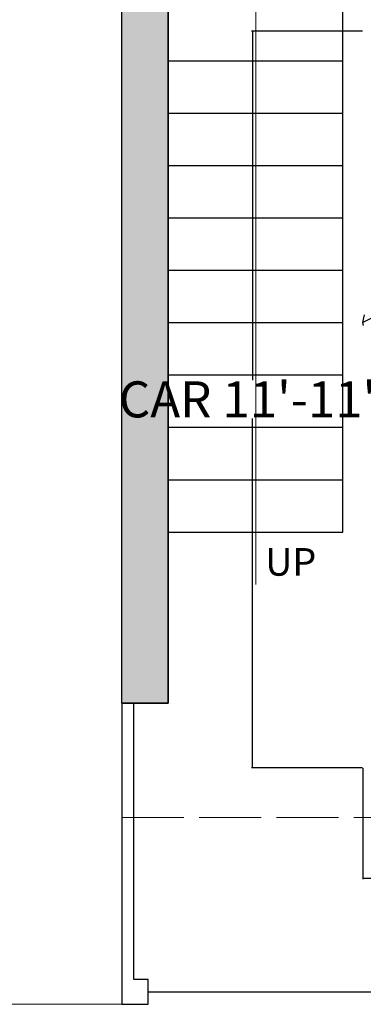
# Model space of a CAD drawing. Units: inches. Extents: x 0 to 4258, y 0 to 3769.
# Tile 3 of 30: x 3659 to 3726, y 2937 to 3128. Entities that reach past the tile are written whole.
import ezdxf

# ---------------------------------------------------------------- set-up
doc = ezdxf.new("R2010")
doc.units = ezdxf.units.IN
doc.header["$MEASUREMENT"] = 0
doc.linetypes.add('ACAD_ISO02W100', pattern=[15, 12, -3])
doc.layers.get('0').update_dxf_attribs({"color": 16})
for name, color, linetype, lineweight in [('A-ANNO-DIMS', 250, 'Continuous', 18), ('A-ANNO-SYMB', 250, 'Continuous', 18), ('A-ANNO-TEXT', 250, 'Continuous', 18), ('A-FLOR-OVHD', 150, 'ACAD_ISO02W100', 13), ('A-FLOR-STRS', 150, 'Continuous', 25), ('A-WALL-PATT', 16, 'Continuous', 13), ('C-PKNG-VEHI', 8, 'Continuous', 18), ('C-PROP', 150, 'Continuous', 25), ('C-ROAD', 250, 'Continuous', 18), ('walls', 251, 'Continuous', 35)]:
    doc.layers.add(name, color=color, linetype=linetype, lineweight=lineweight)
doc.layers.add('Edges', color=250, linetype='Continuous')
doc.styles.get("Standard").update_dxf_attribs({"font": 'arial.ttf'})
doc.dimstyles.get("Standard").update_dxf_attribs({"dimtxt": 7, "dimasz": 0.18, "dimexe": 0.18, "dimexo": 0.0625, "dimgap": 0.09, "dimtad": 0, "dimtih": 1, "dimtoh": 1, "dimzin": 0, "dimdsep": 46, "dimlunit": 3, "dimtxsty": 'Standard', "dimcen": 0.09, "dimadec": 0, "dimazin": 0, "dimtfac": 1, "dimtofl": 0, "dimtmove": 0, "dimatfit": 3, "dimfxl": 1, "dimtolj": 1, "dimtzin": 0, "dimarcsym": 0})

# ---------------------------------------------------------------- blocks, each defined once
blk = doc.blocks.new('Nissan Qashqai pl')
at = {"layer": 'Edges'}
for p, q in [((8.8918, 11.0997), (9.0186, 10.8486)), ((9.0186, 10.8486), (8.9731, 10.8577)), ((9.0374, 10.8517), (9.0186, 10.8486))]:
    blk.add_line(p, q, dxfattribs=at)
blk = doc.blocks.new('car')
blk.add_blockref('Nissan Qashqai pl', (-9.7433, -11.9151))
blk = doc.blocks.new('*D66')
at = {"layer": 'A-ANNO-DIMS', "color": 0, "lineweight": -2, "transparency": 16777216}
for p, q in [((3725.52, 3125.85), (3703.94, 3125.85)), ((3704.12, 3125.67), (3704.12, 3058.01)), ((3704.12, 2982.94), (3704.12, 3050.59)), ((3725.52, 2982.76), (3703.94, 2982.76))]:
    blk.add_line(p, q, dxfattribs=at)
at = {"layer": 'A-ANNO-DIMS', "color": 0, "transparency": 16777216}
for points in [[(3704.09, 3125.67), (3704.15, 3125.67), (3704.12, 3125.85)], [(3704.09, 2982.94), (3704.15, 2982.94), (3704.12, 2982.76)]]:
    blk.add_solid(points, dxfattribs=at)
at = {"layer": 'Defpoints', "color": 0, "transparency": 16777216}
for p in [(3725.58, 3125.85), (3704.12, 2982.76), (3725.58, 2982.76)]:
    blk.add_point(p, dxfattribs=at)
at = {"layer": 'A-ANNO-DIMS', "color": 0, "transparency": 16777216, "insert": (3704.12, 3054.3), "char_height": 7, "attachment_point": 5}
blk.add_mtext('\\A1;CAR 11\'-11"', dxfattribs=at)
blk = doc.blocks.new('*D67')
at = {"layer": 'A-ANNO-DIMS', "color": 0, "lineweight": -2, "transparency": 16777216}
for p, q in [((3725.58, 2982.69), (3725.58, 2961.11)), ((3795.71, 2982.69), (3795.71, 2961.11)), ((3725.76, 2961.29), (3748.53, 2961.29)), ((3795.53, 2961.29), (3772.76, 2961.29))]:
    blk.add_line(p, q, dxfattribs=at)
at = {"layer": 'A-ANNO-DIMS', "color": 0, "transparency": 16777216}
for points in [[(3725.76, 2961.32), (3725.76, 2961.26), (3725.58, 2961.29)], [(3795.53, 2961.32), (3795.53, 2961.26), (3795.71, 2961.29)]]:
    blk.add_solid(points, dxfattribs=at)
at = {"layer": 'Defpoints', "color": 0, "transparency": 16777216}
for p in [(3725.58, 2982.76), (3795.71, 2982.76), (3795.71, 2961.29)]:
    blk.add_point(p, dxfattribs=at)
at = {"layer": 'A-ANNO-DIMS', "color": 0, "transparency": 16777216, "insert": (3760.65, 2961.29), "char_height": 7, "attachment_point": 5}
blk.add_mtext('\\A1;5\'-10"', dxfattribs=at)

msp = doc.modelspace()

# ---------------------------------------------------------------- hatches: boundary and pattern name
at = {"layer": 'A-WALL-PATT'}
h = msp.add_hatch(color=256, dxfattribs=at)
h.dxf.hatch_style = 1
h.paths.add_polyline_path([(3687.804, 3163.293), (3678.804, 3163.293), (3678.804, 2995.293), (3687.804, 2995.293)])
h.paths.add_polyline_path([(3973.039, 3461.793), (3866.304, 3461.793), (3866.304, 3457.293), (3973.039, 3457.293)])
h.paths.add_polyline_path([(4034.304, 3461.793), (4016.474, 3461.793), (4016.474, 3457.293), (4034.304, 3457.293)])

# ---------------------------------------------------------------- linework, layer by layer
at = {"layer": 'A-ANNO-SYMB'}
msp.add_line((3704.8, 3146.777), (3704.8, 3018.327), dxfattribs=at)
at = {"layer": 'A-FLOR-OVHD'}
msp.add_line((3678.804, 2973.052), (3832.744, 2973.052), dxfattribs=at)
at = {"layer": 'A-FLOR-STRS'}
for p, q in [((3721.668, 3028.53), (3721.668, 3163.293)), ((3687.804, 3120.088), (3721.668, 3120.088)), ((3687.804, 3109.915), (3721.668, 3109.915)), ((3687.804, 3099.742), (3721.668, 3099.742)), ((3687.804, 3089.569), (3721.668, 3089.569)), ((3687.804, 3079.396), (3721.668, 3079.396)), ((3687.804, 3069.223), (3721.668, 3069.223)), ((3687.804, 3059.049), (3721.668, 3059.049)), ((3687.804, 3048.876), (3721.668, 3048.876)), ((3687.804, 3038.703), (3721.668, 3038.703)), ((3687.804, 3028.53), (3721.668, 3028.53))]:
    msp.add_line(p, q, dxfattribs=at)
at = {"layer": 'C-PROP'}
for p, q in [((3678.804, 2995.293), (3678.804, 3656.793)), ((3678.804, 2995.293), (3678.804, 2936.793)), ((3681.095, 2941.629), (3681.095, 2995.293)), ((3683.892, 2941.629), (3681.095, 2941.629)), ((3683.892, 2936.793), (3683.892, 2941.629)), ((3683.892, 2939.211), (3766.077, 2939.211)), ((3678.804, 2936.793), (3683.892, 2936.793))]:
    msp.add_line(p, q, dxfattribs=at)
at = {"layer": 'C-ROAD'}
msp.add_line((3678.804, 2936.793), (3596.728, 2936.793), dxfattribs=at)
at = {"layer": 'walls'}
for p, q in [((3687.804, 2995.293), (3687.804, 3163.293)), ((3678.804, 2995.293), (3687.804, 2995.293))]:
    msp.add_line(p, q, dxfattribs=at)

# ---------------------------------------------------------------- block references
at = {"layer": 'C-PKNG-VEHI', "xscale": 32.66500240257601, "yscale": 32.66500240257601, "zscale": 32.66500240257601, "rotation": 270}
msp.add_blockref('car', (3760.419, 3045.57), dxfattribs=at)

# ---------------------------------------------------------------- texts
at = {"layer": 'A-ANNO-TEXT'}
msp.add_text('UP', height=5.3626, dxfattribs=at).set_placement((3706.607, 3020.049))

# ---------------------------------------------------------------- dimensions: what is measured, and where the dimension line sits
at = {"layer": 'A-ANNO-DIMS'}
dim = msp.add_linear_dim(base=(3704.116, 2982.755), p1=(3725.58, 3125.846), p2=(3725.58, 2982.755), angle=270, text='CAR <>', dimstyle='Standard', override={"dimdec": 1, "dimlfac": 1, "dimrnd": 0, "dimzin": 1, "dimdsep": 46, "dimlunit": 4, "dimfrac": 2}, dxfattribs=at)
dim.commit()
dim.dimension.update_dxf_attribs({"geometry": '*D66', "text_midpoint": (3704.116, 3054.301)})
dim = msp.add_linear_dim(base=(3795.713, 2961.292), p1=(3725.58, 2982.755), p2=(3795.713, 2982.755), dimstyle='Standard', override={"dimdec": 1, "dimlfac": 1, "dimrnd": 0, "dimzin": 1, "dimdsep": 46, "dimlunit": 4, "dimfrac": 2}, dxfattribs=at)
dim.commit()
dim.dimension.update_dxf_attribs({"geometry": '*D67', "text_midpoint": (3760.646, 2961.292)})

doc.saveas('drawing.dxf')
